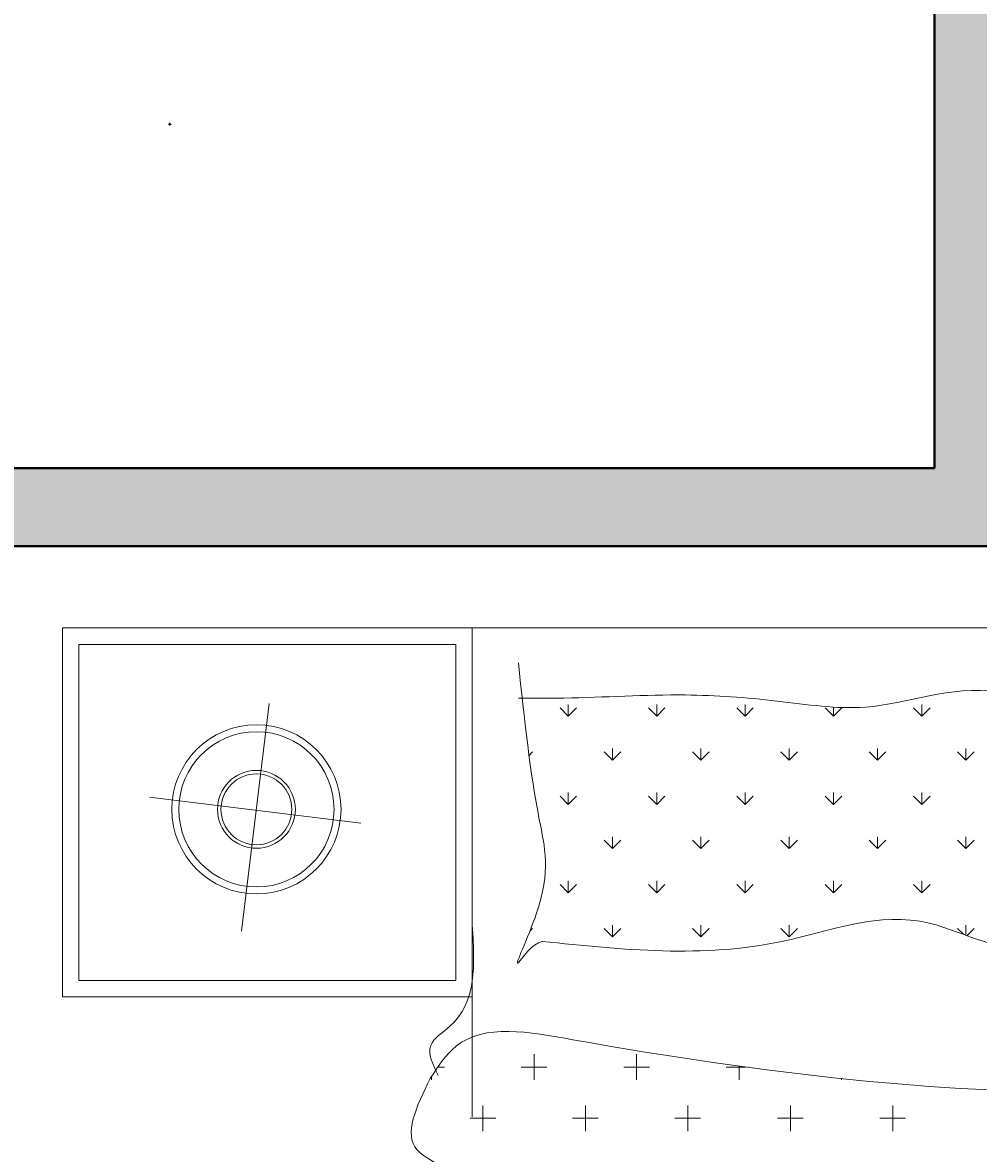
# Model space of a CAD drawing. Units: inches. Extents: x 2330 to 3943, y 1763 to 3461.
# Tile 19 of 40: x 3096 to 3157, y 2662 to 2734. Entities that reach past the tile are written whole.
import ezdxf

# ---------------------------------------------------------------- set-up
doc = ezdxf.new("R2010")
doc.units = ezdxf.units.IN
for name, color, linetype, lineweight in [('A-ANNO-DIMS', 2, 'Continuous', 18), ('A-FURN', 8, 'Continuous', 13), ('A-WALL', 7, 'Continuous', 40), ('A-WALL-PATT', 252, 'Continuous', 13)]:
    doc.layers.add(name, color=color, linetype=linetype, lineweight=lineweight)
doc.styles.get("Standard").update_dxf_attribs({"font": 'arial.ttf'})
doc.dimstyles.get("Standard").update_dxf_attribs({"dimtxt": 0.18, "dimasz": 0.18, "dimexe": 0.18, "dimexo": 0.0625, "dimgap": 0.09, "dimtad": 0, "dimtih": 1, "dimtoh": 1, "dimdec": 4, "dimzin": 0, "dimdsep": 46, "dimtxsty": 'Standard', "dimcen": 0.09, "dimadec": 0, "dimazin": 0, "dimtfac": 1, "dimtdec": 4, "dimtofl": 0, "dimtmove": 0, "dimatfit": 3, "dimfxl": 1, "dimtolj": 1, "dimtzin": 0, "dimarcsym": 0})

# ---------------------------------------------------------------- blocks, each defined once
blk = doc.blocks.new('A$C200C7901')
for p, q in [((0, 1.8834), (0, 2.3334)), ((0.5, 2.3334), (0, 2.3334)), ((0.5, 2.3334), (0.5, 1.7369)), ((0.5, 2.3334), (0.5, 1.7369)), ((0.5, 2.3334), (2, 2.3334)), ((0.9943, 2.1721), (0.9842, 2.1822)), ((0.9943, 2.1721), (0.9842, 2.1822)), ((0.9943, 2.0643), (0.9842, 2.0744)), ((0.9943, 2.0643), (0.9842, 2.0744)), ((0.5701, 1.9635), (0.5733, 1.9666)), ((0.5701, 1.9635), (0.5733, 1.9666)), ((0.5, 1.8834), (0, 1.8834)), ((0.458, 1.7977), (0.466, 1.7977)), ((0.458, 1.7977), (0.466, 1.7977)), ((0.4504, 1.782), (0.4504, 1.7863)), ((0.4504, 1.782), (0.4504, 1.7863))]:
    blk.add_line(p, q)
at = {"linetype": 'ByBlock'}
for p, q in [((0.02, 1.9034), (0.02, 2.3134)), ((0.48, 2.3134), (0.02, 2.3134)), ((0.48, 1.9034), (0.48, 2.3134)), ((0.2524, 2.2412), (0.2186, 1.9635)), ((0.6171, 2.2259), (0.607, 2.236)), ((0.6171, 2.2259), (0.607, 2.236)), ((0.6171, 2.2259), (0.6171, 2.2402)), ((0.6171, 2.2259), (0.6171, 2.2402)), ((0.6171, 2.2259), (0.6272, 2.236)), ((0.6171, 2.2259), (0.6272, 2.236)), ((0.7249, 2.2259), (0.7148, 2.236)), ((0.7249, 2.2259), (0.7148, 2.236)), ((0.7249, 2.2259), (0.7249, 2.2402)), ((0.7249, 2.2259), (0.7249, 2.2402)), ((0.7249, 2.2259), (0.735, 2.236)), ((0.7249, 2.2259), (0.735, 2.236)), ((0.8326, 2.2259), (0.8225, 2.236)), ((0.8326, 2.2259), (0.8225, 2.236)), ((0.8326, 2.2259), (0.8326, 2.2402)), ((0.8326, 2.2259), (0.8326, 2.2402)), ((0.8326, 2.2259), (0.8427, 2.236)), ((0.8326, 2.2259), (0.8427, 2.236)), ((0.9404, 2.2259), (0.9303, 2.236)), ((0.9404, 2.2259), (0.9303, 2.236)), ((0.9404, 2.2259), (0.9404, 2.2369)), ((0.9404, 2.2259), (0.9404, 2.2369)), ((0.9404, 2.2259), (0.9505, 2.236)), ((0.9404, 2.2259), (0.9505, 2.236)), ((1.0482, 2.2259), (1.0381, 2.236)), ((1.0482, 2.2259), (1.0381, 2.236)), ((1.0482, 2.2259), (1.0482, 2.2402)), ((1.0482, 2.2259), (1.0482, 2.2402)), ((1.0482, 2.2259), (1.0583, 2.236)), ((1.0482, 2.2259), (1.0583, 2.236)), ((0.5692, 2.178), (0.5733, 2.1822)), ((0.5692, 2.178), (0.5733, 2.1822)), ((0.671, 2.1721), (0.6609, 2.1822)), ((0.671, 2.1721), (0.6609, 2.1822)), ((0.671, 2.172), (0.671, 2.1863)), ((0.671, 2.172), (0.671, 2.1863)), ((0.671, 2.1721), (0.6811, 2.1822)), ((0.671, 2.1721), (0.6811, 2.1822)), ((0.7787, 2.1721), (0.7686, 2.1822)), ((0.7787, 2.1721), (0.7686, 2.1822)), ((0.7787, 2.172), (0.7787, 2.1863)), ((0.7787, 2.172), (0.7787, 2.1863)), ((0.7787, 2.1721), (0.7889, 2.1822)), ((0.7787, 2.1721), (0.7889, 2.1822)), ((0.8865, 2.1721), (0.8764, 2.1822)), ((0.8865, 2.1721), (0.8764, 2.1822)), ((0.8865, 2.172), (0.8865, 2.1863)), ((0.8865, 2.172), (0.8865, 2.1863)), ((0.8865, 2.1721), (0.8966, 2.1822)), ((0.8865, 2.1721), (0.8966, 2.1822)), ((0.9943, 2.172), (0.9943, 2.1863)), ((0.9943, 2.172), (0.9943, 2.1863)), ((0.9943, 2.1721), (1.0044, 2.1822)), ((0.9943, 2.1721), (1.0044, 2.1822)), ((1.102, 2.1721), (1.0919, 2.1822)), ((1.102, 2.1721), (1.0919, 2.1822)), ((1.102, 2.172), (1.102, 2.1863)), ((1.102, 2.172), (1.102, 2.1863)), ((1.102, 2.1721), (1.1121, 2.1822)), ((1.102, 2.1721), (1.1121, 2.1822)), ((0.3641, 2.0951), (0.1061, 2.1268)), ((0.6171, 2.1182), (0.607, 2.1283)), ((0.6171, 2.1182), (0.607, 2.1283)), ((0.6171, 2.1182), (0.6171, 2.1325)), ((0.6171, 2.1182), (0.6171, 2.1325)), ((0.6171, 2.1182), (0.6272, 2.1283)), ((0.6171, 2.1182), (0.6272, 2.1283)), ((0.7249, 2.1182), (0.7148, 2.1283)), ((0.7249, 2.1182), (0.7148, 2.1283)), ((0.7249, 2.1182), (0.7249, 2.1325)), ((0.7249, 2.1182), (0.7249, 2.1325)), ((0.7249, 2.1182), (0.735, 2.1283)), ((0.7249, 2.1182), (0.735, 2.1283)), ((0.8326, 2.1182), (0.8225, 2.1283)), ((0.8326, 2.1182), (0.8225, 2.1283)), ((0.8326, 2.1182), (0.8326, 2.1325)), ((0.8326, 2.1182), (0.8326, 2.1325)), ((0.8326, 2.1182), (0.8427, 2.1283)), ((0.8326, 2.1182), (0.8427, 2.1283)), ((0.9404, 2.1182), (0.9303, 2.1283)), ((0.9404, 2.1182), (0.9303, 2.1283)), ((0.9404, 2.1182), (0.9404, 2.1325)), ((0.9404, 2.1182), (0.9404, 2.1325)), ((0.9404, 2.1182), (0.9505, 2.1283)), ((0.9404, 2.1182), (0.9505, 2.1283)), ((1.0482, 2.1182), (1.0381, 2.1283)), ((1.0482, 2.1182), (1.0381, 2.1283)), ((1.0482, 2.1182), (1.0482, 2.1325)), ((1.0482, 2.1182), (1.0482, 2.1325)), ((1.0482, 2.1182), (1.0583, 2.1283)), ((1.0482, 2.1182), (1.0583, 2.1283)), ((0.671, 2.0643), (0.6609, 2.0744)), ((0.671, 2.0643), (0.6609, 2.0744)), ((0.671, 2.0643), (0.671, 2.0786)), ((0.671, 2.0643), (0.671, 2.0786)), ((0.671, 2.0643), (0.6811, 2.0744)), ((0.671, 2.0643), (0.6811, 2.0744)), ((0.7787, 2.0643), (0.7686, 2.0744)), ((0.7787, 2.0643), (0.7686, 2.0744)), ((0.7787, 2.0643), (0.7787, 2.0786)), ((0.7787, 2.0643), (0.7787, 2.0786)), ((0.7787, 2.0643), (0.7889, 2.0744)), ((0.7787, 2.0643), (0.7889, 2.0744)), ((0.8865, 2.0643), (0.8764, 2.0744)), ((0.8865, 2.0643), (0.8764, 2.0744)), ((0.8865, 2.0643), (0.8865, 2.0786)), ((0.8865, 2.0643), (0.8865, 2.0786)), ((0.8865, 2.0643), (0.8966, 2.0744)), ((0.8865, 2.0643), (0.8966, 2.0744)), ((0.9943, 2.0643), (0.9943, 2.0786)), ((0.9943, 2.0643), (0.9943, 2.0786)), ((0.9943, 2.0643), (1.0044, 2.0744)), ((0.9943, 2.0643), (1.0044, 2.0744)), ((1.102, 2.0643), (1.0919, 2.0744)), ((1.102, 2.0643), (1.0919, 2.0744)), ((1.102, 2.0643), (1.102, 2.0786)), ((1.102, 2.0643), (1.102, 2.0786)), ((1.102, 2.0643), (1.1121, 2.0744)), ((1.102, 2.0643), (1.1121, 2.0744)), ((0.6171, 2.0104), (0.607, 2.0205)), ((0.6171, 2.0104), (0.607, 2.0205)), ((0.6171, 2.0104), (0.6171, 2.0247)), ((0.6171, 2.0104), (0.6171, 2.0247)), ((0.6171, 2.0104), (0.6272, 2.0205)), ((0.6171, 2.0104), (0.6272, 2.0205)), ((0.7249, 2.0104), (0.7148, 2.0205)), ((0.7249, 2.0104), (0.7148, 2.0205)), ((0.7249, 2.0104), (0.7249, 2.0247)), ((0.7249, 2.0104), (0.7249, 2.0247)), ((0.7249, 2.0104), (0.735, 2.0205)), ((0.7249, 2.0104), (0.735, 2.0205)), ((0.8326, 2.0104), (0.8225, 2.0205)), ((0.8326, 2.0104), (0.8225, 2.0205)), ((0.8326, 2.0104), (0.8326, 2.0247)), ((0.8326, 2.0104), (0.8326, 2.0247)), ((0.8326, 2.0104), (0.8427, 2.0205)), ((0.8326, 2.0104), (0.8427, 2.0205)), ((0.9404, 2.0104), (0.9303, 2.0205)), ((0.9404, 2.0104), (0.9303, 2.0205)), ((0.9404, 2.0104), (0.9404, 2.0247)), ((0.9404, 2.0104), (0.9404, 2.0247)), ((0.9404, 2.0104), (0.9505, 2.0205)), ((0.9404, 2.0104), (0.9505, 2.0205)), ((1.0482, 2.0104), (1.0381, 2.0205)), ((1.0482, 2.0104), (1.0381, 2.0205)), ((1.0482, 2.0104), (1.0482, 2.0247)), ((1.0482, 2.0104), (1.0482, 2.0247)), ((1.0482, 2.0104), (1.0583, 2.0205)), ((1.0482, 2.0104), (1.0583, 2.0205)), ((0.671, 1.9565), (0.6609, 1.9666)), ((0.671, 1.9565), (0.6609, 1.9666)), ((0.671, 1.9565), (0.671, 1.9708)), ((0.671, 1.9565), (0.671, 1.9708)), ((0.671, 1.9565), (0.6811, 1.9666)), ((0.671, 1.9565), (0.6811, 1.9666)), ((0.7787, 1.9565), (0.7686, 1.9666)), ((0.7787, 1.9565), (0.7686, 1.9666)), ((0.7787, 1.9565), (0.7787, 1.9708)), ((0.7787, 1.9565), (0.7787, 1.9708)), ((0.7787, 1.9565), (0.7889, 1.9666)), ((0.7787, 1.9565), (0.7889, 1.9666)), ((0.8865, 1.9565), (0.8764, 1.9666)), ((0.8865, 1.9565), (0.8764, 1.9666)), ((0.8865, 1.9565), (0.8865, 1.9708)), ((0.8865, 1.9565), (0.8865, 1.9708)), ((0.8865, 1.9565), (0.8966, 1.9666)), ((0.8865, 1.9565), (0.8966, 1.9666)), ((1.0993, 1.9593), (1.0919, 1.9666)), ((1.0993, 1.9593), (1.0919, 1.9666)), ((1.102, 1.9583), (1.102, 1.9708)), ((1.102, 1.9583), (1.102, 1.9708)), ((1.1033, 1.9578), (1.1121, 1.9666)), ((1.1033, 1.9578), (1.1121, 1.9666)), ((0.48, 1.9034), (0.02, 1.9034)), ((0.5754, 1.782), (0.5754, 1.8133)), ((0.5754, 1.782), (0.5754, 1.8133)), ((0.7004, 1.782), (0.7004, 1.8133)), ((0.7004, 1.782), (0.7004, 1.8133)), ((0.5597, 1.7977), (0.591, 1.7977)), ((0.5597, 1.7977), (0.591, 1.7977)), ((0.6847, 1.7977), (0.716, 1.7977)), ((0.6847, 1.7977), (0.716, 1.7977)), ((0.8097, 1.7977), (0.8331, 1.7977)), ((0.8097, 1.7977), (0.8331, 1.7977)), ((0.8254, 1.782), (0.8254, 1.7987)), ((0.8254, 1.782), (0.8254, 1.7987)), ((0.9504, 1.782), (0.9504, 1.7836)), ((0.9504, 1.782), (0.9504, 1.7836)), ((0.5129, 1.7195), (0.5129, 1.7508)), ((0.5129, 1.7195), (0.5129, 1.7508)), ((0.6379, 1.7195), (0.6379, 1.7508)), ((0.6379, 1.7195), (0.6379, 1.7508)), ((0.7629, 1.7195), (0.7629, 1.7508)), ((0.7629, 1.7195), (0.7629, 1.7508)), ((0.8879, 1.7195), (0.8879, 1.7508)), ((0.8879, 1.7195), (0.8879, 1.7508)), ((1.0129, 1.7195), (1.0129, 1.7508)), ((1.0129, 1.7195), (1.0129, 1.7508)), ((0.4972, 1.7352), (0.5285, 1.7352)), ((0.4972, 1.7352), (0.5285, 1.7352)), ((0.6222, 1.7352), (0.6535, 1.7352)), ((0.6222, 1.7352), (0.6535, 1.7352)), ((0.7472, 1.7352), (0.7785, 1.7352)), ((0.7472, 1.7352), (0.7785, 1.7352)), ((0.8722, 1.7352), (0.9035, 1.7352)), ((0.8722, 1.7352), (0.9035, 1.7352)), ((0.9972, 1.7352), (1.0285, 1.7352)), ((0.9972, 1.7352), (1.0285, 1.7352))]:
    blk.add_line(p, q, dxfattribs=at)
for radius in [0.1032, 0.0947, 0.0475, 0.0432]:
    blk.add_circle((0.2367, 2.1121), radius, dxfattribs=at)
for points, knots in [([(0.5562, 2.2908), (0.5634, 2.223), (0.5751, 2.1147), (0.6005, 2.0213), (0.5392, 1.8966), (0.5726, 1.9486), (0.5854, 1.951)], [0, 0, 0, 0, 193.119101, 308.278592, 371.468985, 410.593498, 410.593498, 410.593498, 410.593498]), ([(0.5854, 1.951), (0.6835, 1.9407), (0.8425, 1.9242), (1.0374, 2.0054), (1.1564, 1.9255), (1.2274, 1.9841), (1.2052, 2.0751), (1.1815, 2.152), (1.2176, 2.2368), (1.0992, 2.2731), (1.0008, 2.2255), (0.8698, 2.246), (0.7481, 2.2548), (0.6426, 2.2473), (0.5746, 2.2478), (0.5562, 2.2479)], [0, 0, 0, 0, 292.165466, 473.33038, 601.631673, 630.723769, 727.138505, 836.819956, 887.958136, 954.42438, 1118.989809, 1227.016542, 1338.750986, 1487.447361, 1542.751028, 1542.751028, 1542.751028, 1542.751028]), ([(0.4485, 1.7835), (0.4321, 1.7496), (0.4062, 1.6964), (0.49, 1.6713), (0.4719, 1.5969), (0.4123, 1.592), (0.4233, 1.5337), (0.4954, 1.5086), (0.4012, 1.4738), (0.3253, 1.4306), (0.4113, 1.3764), (0.3688, 1.3065), (0.5579, 1.2663), (0.741, 1.4533), (1.1127, 1.1109), (1.4811, 1.2478), (1.7885, 1.3492), (2.0357, 1.1637), (2.0748, 1.2974), (2.0876, 1.349), (2.0192, 1.3805), (2.0564, 1.4298), (2.0588, 1.4846), (1.9759, 1.5349), (2.1004, 1.5845), (2.0397, 1.6519), (1.971, 1.7053), (2.1104, 1.8981), (1.5946, 1.7967), (1.2448, 1.7472), (0.8129, 1.7935), (0.4953, 1.8548), (0.4582, 1.7983), (0.4485, 1.7835)], [0, 0, 0, 0, 88.420092, 139.08588, 204.302936, 239.695496, 287.801042, 327.365471, 412.960499, 463.626286, 552.059846, 584.668336, 662.614915, 940.993281, 1309.926334, 1844.022653, 1996.276242, 2316.43048, 2341.441004, 2404.707416, 2449.463774, 2514.680778, 2538.40571, 2613.031547, 2697.13096, 2760.903931, 2822.692699, 2945.47, 3215.060018, 3725.584917, 4361.974444, 4504.671998, 4555.32777, 4555.32777, 4555.32777, 4555.32777])]:
    blk.add_open_spline(points, degree=3, knots=knots)
blk.add_open_spline([(0.5, 1.9703), (0.5029, 1.9235), (0.5066, 1.8648), (0.4398, 1.8252), (0.452, 1.8005), (0.4585, 1.7872)], degree=3, knots=[0, 0, 0, 0, 126.315232, 158.854004, 196.789047, 196.789047, 196.789047, 196.789047], dxfattribs=at)
blk.add_open_spline([(0.5, 1.9703), (0.5029, 1.9235), (0.5066, 1.8648), (0.4398, 1.8252), (0.452, 1.8005), (0.4585, 1.7872)], degree=3, knots=[0, 0, 0, 0, 126.315232, 158.854004, 196.789047, 196.789047, 196.789047, 196.789047], dxfattribs=at)
blk = doc.blocks.new('*D95')
at = {"layer": 'A-ANNO-DIMS', "color": 0, "lineweight": -2, "transparency": 16777216}
for p, q in [((3105.603, 2727.687), (3105.783, 2727.687)), ((3105.693, 2727.597), (3105.693, 2727.777)), ((3606.312, 2659.69), (3418.758, 2685.165))]:
    blk.add_line(p, q, dxfattribs=at)
at = {"layer": 'A-ANNO-DIMS', "color": 0, "transparency": 16777216}
blk.add_solid([(3418.762, 2685.195), (3418.754, 2685.135), (3418.58, 2685.189)], dxfattribs=at)
at = {"layer": 'Defpoints', "color": 0, "transparency": 16777216}
for p in [(3105.693, 2727.687), (3418.58, 2685.189)]:
    blk.add_point(p, dxfattribs=at)
at = {"layer": 'A-ANNO-DIMS', "color": 0, "transparency": 16777216, "insert": (3606.862, 2659.69), "char_height": 0.18, "attachment_point": 5}
blk.add_mtext('\\A1;R315.76', dxfattribs=at)
blk = doc.blocks.new('*D96')
at = {"layer": 'A-ANNO-DIMS', "color": 0, "lineweight": -2, "transparency": 16777216}
for p, q in [((3604.649, 2753.345), (3417.721, 2743.732)), ((3105.603, 2727.687), (3105.783, 2727.687)), ((3105.693, 2727.597), (3105.693, 2727.777))]:
    blk.add_line(p, q, dxfattribs=at)
at = {"layer": 'A-ANNO-DIMS', "color": 0, "transparency": 16777216}
blk.add_solid([(3417.719, 2743.762), (3417.722, 2743.702), (3417.541, 2743.723)], dxfattribs=at)
at = {"layer": 'Defpoints', "color": 0, "transparency": 16777216}
for p in [(3417.541, 2743.723), (3105.693, 2727.687)]:
    blk.add_point(p, dxfattribs=at)
at = {"layer": 'A-ANNO-DIMS', "color": 0, "transparency": 16777216, "insert": (3605.394, 2753.345), "char_height": 0.18, "attachment_point": 5}
blk.add_mtext('\\A1;2X R312.26', dxfattribs=at)
blk = doc.blocks.new('*D97')
at = {"layer": 'A-ANNO-DIMS', "color": 0, "lineweight": -2, "transparency": 16777216}
for p, q in [((3105.603, 2727.687), (3105.783, 2727.687)), ((3105.693, 2727.597), (3105.693, 2727.777)), ((3589.166, 2615.071), (3408.039, 2657.261))]:
    blk.add_line(p, q, dxfattribs=at)
at = {"layer": 'A-ANNO-DIMS', "color": 0, "transparency": 16777216}
blk.add_solid([(3408.046, 2657.29), (3408.032, 2657.232), (3407.864, 2657.302)], dxfattribs=at)
at = {"layer": 'Defpoints', "color": 0, "transparency": 16777216}
for p in [(3105.693, 2727.687), (3407.864, 2657.302)]:
    blk.add_point(p, dxfattribs=at)
at = {"layer": 'A-ANNO-DIMS', "color": 0, "transparency": 16777216, "insert": (3589.911, 2615.071), "char_height": 0.18, "attachment_point": 5}
blk.add_mtext('\\A1;2X R310.26', dxfattribs=at)
blk = doc.blocks.new('*D98')
at = {"layer": 'A-ANNO-DIMS', "color": 0, "lineweight": -2, "transparency": 16777216}
for p, q in [((3105.603, 2727.687), (3105.783, 2727.687)), ((3105.693, 2727.597), (3105.693, 2727.777)), ((3519.334, 2463.489), (3364.371, 2562.466)), ((3519.514, 2463.489), (3519.334, 2463.489))]:
    blk.add_line(p, q, dxfattribs=at)
at = {"layer": 'A-ANNO-DIMS', "color": 0, "transparency": 16777216}
blk.add_solid([(3364.387, 2562.491), (3364.355, 2562.441), (3364.219, 2562.563)], dxfattribs=at)
at = {"layer": 'Defpoints', "color": 0, "transparency": 16777216}
for p in [(3105.693, 2727.687), (3364.219, 2562.563)]:
    blk.add_point(p, dxfattribs=at)
at = {"layer": 'A-ANNO-DIMS', "color": 0, "transparency": 16777216, "insert": (3520.257, 2463.489), "char_height": 0.18, "attachment_point": 5}
blk.add_mtext('\\A1;3X R306.76', dxfattribs=at)

msp = doc.modelspace()

# ---------------------------------------------------------------- hatches: boundary and pattern name
at = {"layer": 'A-WALL-PATT'}
h = msp.add_hatch(color=256, dxfattribs=at)
h.dxf.hatch_style = 1
h.paths.add_polyline_path([(3420.6832, 2705.6524), (3159.6605, 2705.6524), (3159.6605, 2827.6524), (3154.6605, 2827.6524), (3154.6605, 2705.6524), (3017.6605, 2705.6524), (3017.6605, 2700.6524), (3238.6605, 2700.6524), (3238.6605, 2605.6524), (3247.6605, 2605.6524), (3247.6605, 2610.6524), (3243.6605, 2610.6524), (3243.6605, 2700.6524), (3411.2593, 2700.6524, -0.0252833), (3406.9698, 2669.9468), (3415.809, 2668.2528, 0.029888)])

# ---------------------------------------------------------------- linework, layer by layer
at = {"layer": 'A-WALL'}
for p, q in [((3154.6605, 2827.6524), (3154.6605, 2705.6524)), ((3017.6605, 2705.6524), (3154.6605, 2705.6524)), ((3017.6605, 2700.6524), (3238.6605, 2700.6524))]:
    msp.add_line(p, q, dxfattribs=at)

# ---------------------------------------------------------------- block references
at = {"layer": 'A-FURN', "xscale": 52.5181391560459, "yscale": 52.5181391560459, "zscale": 52.5181391560459}
msp.add_blockref('A$C200C7901', (3098.8053, 2572.8601), dxfattribs=at)

# ---------------------------------------------------------------- dimensions: what is measured, and where the dimension line sits
at = {"layer": 'A-ANNO-DIMS'}
for mpoint, text, picture, middle in [((3417.5409, 2743.723), '2X <>', '*D96', (3604.6494, 2753.3446)), ((3407.8638, 2657.302), '2X <>', '*D97', (3589.166, 2615.0711)), ((3364.219, 2562.563), '3X <>', '*D98', (3520.2574, 2463.4886))]:
    dim = msp.add_radius_dim(center=(3105.6935, 2727.6869), mpoint=mpoint, text=text, dimstyle='Standard', override={"dimdec": 2, "dimlfac": 1, "dimrnd": 0, "dimzin": 0, "dimdsep": 46, "dimlunit": 2}, dxfattribs=at)
    dim.commit()
    dim.dimension.update_dxf_attribs({"geometry": picture, "text_midpoint": middle, "dimtype": 164})
dim = msp.add_radius_dim(center=(3105.6935, 2727.6869), mpoint=(3418.58, 2685.189), dimstyle='Standard', override={"dimdec": 2, "dimlfac": 1, "dimrnd": 0, "dimzin": 0, "dimdsep": 46, "dimlunit": 2}, dxfattribs=at)
dim.commit()
dim.dimension.update_dxf_attribs({"geometry": '*D95', "text_midpoint": (3606.3119, 2659.6902), "dimtype": 164})

doc.saveas('drawing.dxf')
